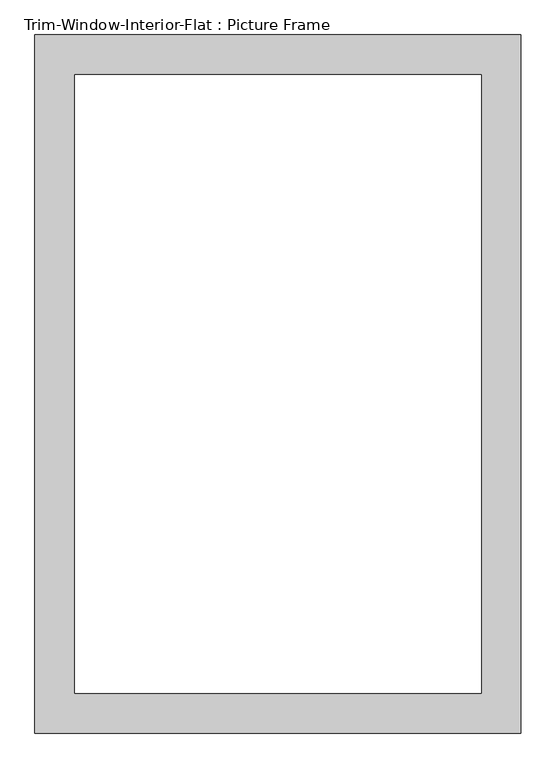
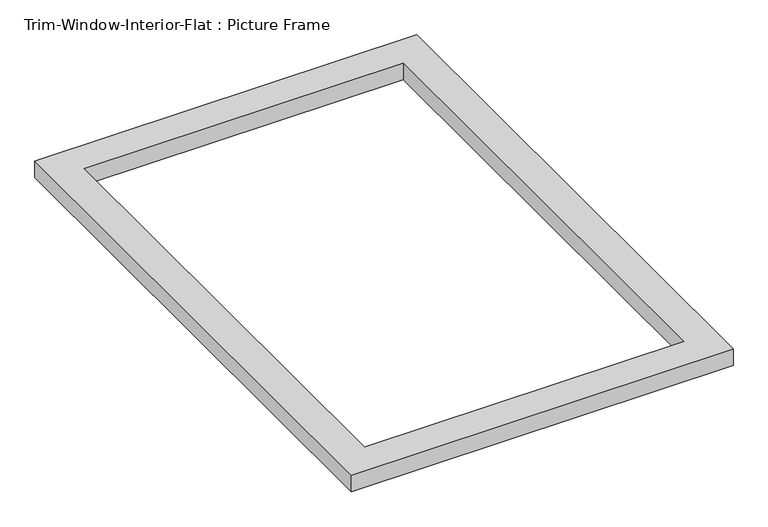
"""IFC4 building model written with IfcOpenShell, lengths in millimetres: proxy geometry, Trim-Window-Interior-Flat : Picture Frame."""

from ifc_helpers import new_model, si_unit, origin, origin_with_axes, place, context, project, spatial, polyline, outline, extrude, source, transform, mapped, element, save


def trim_window_interior_flat_picture_frame_d485c387(model_context):
    return source(origin(), model_context, "Body", "SweptSolid", [
        extrude(outline(polyline([(349.25, 44.45), (349.25, -958.85), (-349.25, -958.85), (-349.25, 44.45), (349.25, 44.45)]), holes=[polyline([(292.1, -12.7), (-292.1, -12.7), (-292.1, -901.7), (292.1, -901.7), (292.1, -12.7)])]), origin_with_axes(), (0.0, 0.0, 1.0), 31.75),
    ])


if __name__ == "__main__":
    model = new_model("IFC4")
    model_context = context("Model", 3, world=origin())
    ifc_project = project(units=[si_unit("LENGTHUNIT", "METRE", prefix="MILLI")], contexts=[model_context])
    site = spatial("IfcSite", under=ifc_project)
    building = spatial("IfcBuilding", under=site)
    placement = place(None, origin())
    trim_window_interior_flat_picture_frame_shape = trim_window_interior_flat_picture_frame_d485c387(model_context)
    element("IfcBuildingElementProxy", 1, Name="Trim-Window-Interior-Flat : Picture Frame", ObjectType="Trim-Window-Interior-Flat : Picture Frame", at=placement, inside=building, context=model_context, shape_type="MappedRepresentation", body=[
        mapped(trim_window_interior_flat_picture_frame_shape, transform((0.0, 0.0, 0.0), x_axis=(1.0, 0.0, 0.0), y_axis=(0.0, 1.0, 0.0), z_axis=(0.0, 0.0, 1.0))),
    ])
    save(model, "model.ifc")

# Revit data of these elements
# Type "Trim-Window-Interior-Flat : Picture Frame"
#   Trim Thickness_Picture Frame = 0' - 1 1/4"
#   Trim Width = 0' - 2 1/4"
#   Trim Thickness_with Sill = 0' - 0 3/4"
#   Sill Thickness = 0' - 1 1/4"
#   Opening Width [instance default] = 2' - 0"
#   Opening Height [instance default] = 3' - 0"
#   Default Elevation = 4' - 0"
#   Sill = no
#   Picture Frame = yes
#   Trim Material [instance default] = none
# Element 1 (IfcBuildingElementProxy, "Trim-Window-Interior-Flat : Picture Frame")
#   Trim Material = Wood - Stained
#   Materials on its faces: "Wood - Stained"
# Materials
#   "Wood - Stained": class "Wood", colour RGB 173 132 96, transparency 0, Cost = 0
